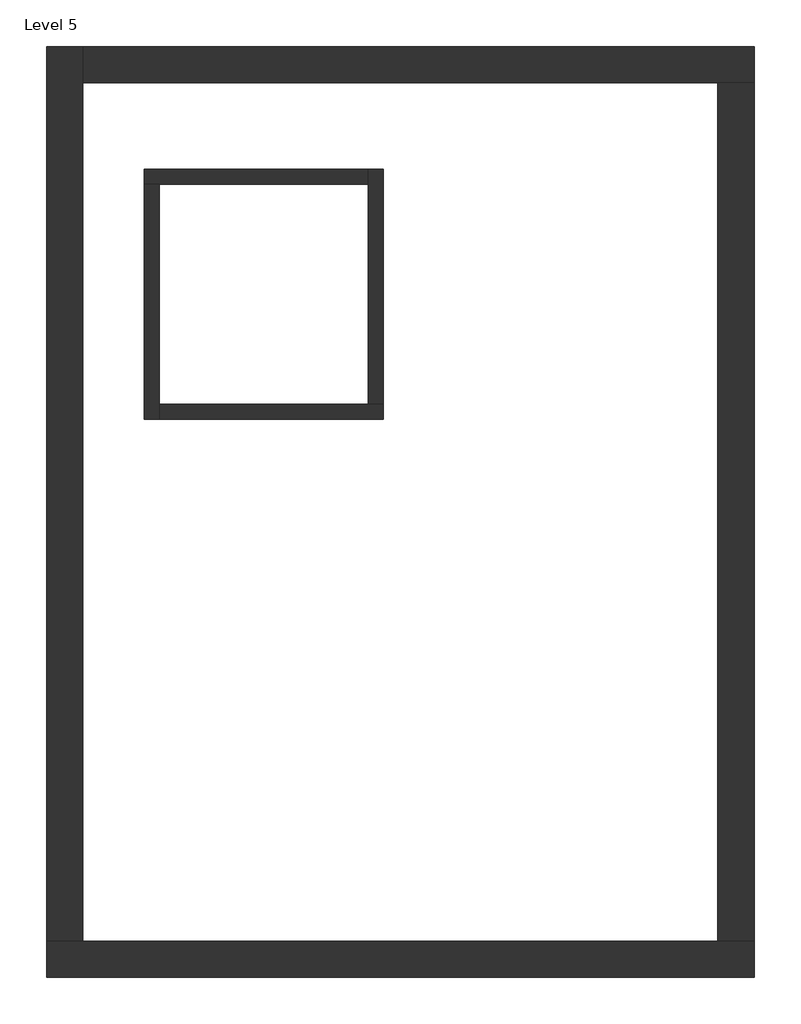
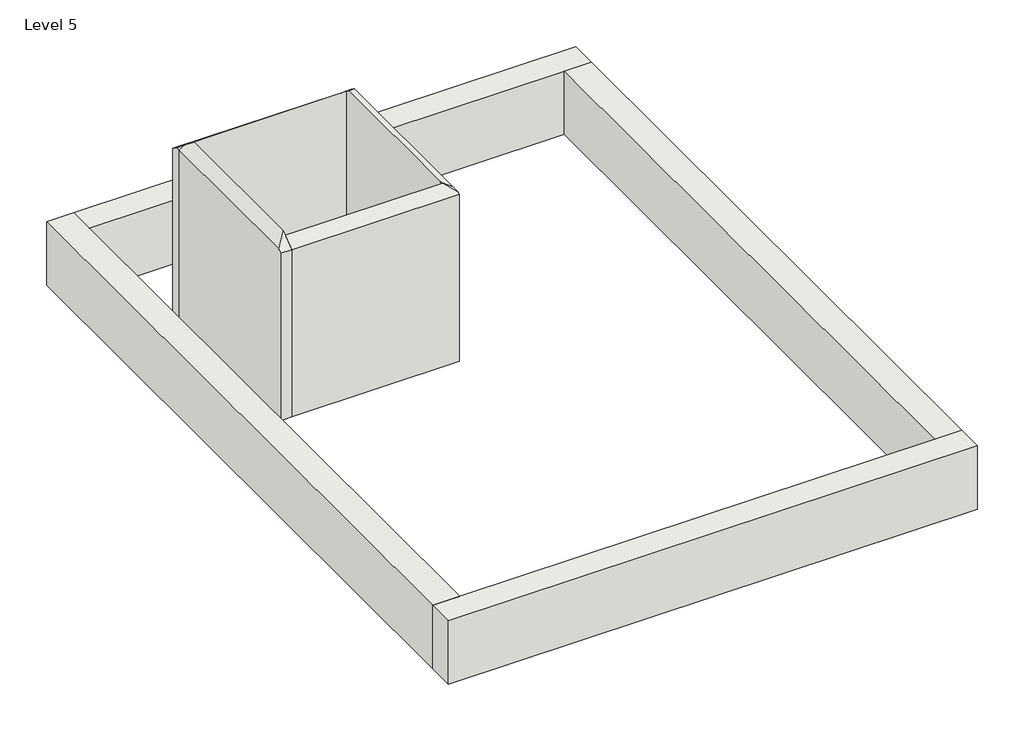
# One storey: 8 walls.
"""IFC4 building model written with IfcOpenShell, lengths in millimetres."""

from ifc_helpers import new_model, si_unit, frame, origin, place, context, project, spatial, polyline, outline, extrude, faceted_brep, element, save

model = new_model("IFC4")

# Units and contexts
model_context = context("Model", 3, world=origin())
ifc_project = project(units=[si_unit("LENGTHUNIT", "METRE", prefix="MILLI")], contexts=[model_context])

# Site, building, storey
site = spatial("IfcSite", under=ifc_project)
building = spatial("IfcBuilding", under=site)
storey = spatial("IfcBuildingStorey", under=building, Name="Level 5", Elevation=6553.2)

# Walls
placement = place(None, origin())
element("IfcWall", 1, ObjectType="Exterior - Brick on CMU", at=placement, inside=storey, context=model_context, shape_type="Brep", body=[
    faceted_brep([(-1013.5628458, 2205.3847306, 6553.2), (-1508.8628458, 2205.3847306, 6553.2), (-10157.5628458, 2205.3847306, 6553.2), (-10652.8628458, 2205.3847306, 6553.2), (-10652.8628458, 2205.3847306, 7772.4), (-10157.5628458, 2205.3847306, 7772.4), (-1508.8628458, 2205.3847306, 7772.4), (-1013.5628458, 2205.3847306, 7772.4), (-1013.5628458, 1710.0847306, 6553.2), (-1013.5628458, 1710.0847306, 7772.4), (-10652.8628458, 1710.0847306, 7772.4), (-10652.8628458, 1710.0847306, 6553.2)], [[[0, 1, 2, 3, 4, 5, 6, 7]], [[8, 9, 10, 11]], [[3, 2, 1, 0, 8, 11]], [[7, 6, 5, 4, 10, 9]], [[4, 3, 11, 10]], [[0, 7, 9, 8]]]),
])
element("IfcWall", 2, ObjectType="Exterior - Brick on CMU", at=placement, inside=storey, context=model_context, shape_type="Brep", body=[
    faceted_brep([(-10157.5628458, 2205.3847306, 6553.2), (-10157.5628458, 13897.569734, 6553.2), (-10157.5628458, 14392.869734, 6553.2), (-10157.5628458, 14392.869734, 7772.4), (-10157.5628458, 13897.569734, 7772.4), (-10157.5628458, 2205.3847306, 7772.4), (-10652.8628458, 2205.3847306, 6553.2), (-10652.8628458, 2205.3847306, 7772.4), (-10652.8628458, 14392.869734, 7772.4), (-10652.8628458, 14392.869734, 6553.2)], [[[0, 1, 2, 3, 4, 5]], [[6, 7, 8, 9]], [[2, 1, 0, 6, 9]], [[5, 4, 3, 8, 7]], [[0, 5, 7, 6]], [[3, 2, 9, 8]]]),
])
element("IfcWall", 3, ObjectType="Exterior - Brick on CMU", at=placement, inside=storey, context=model_context, shape_type="Brep", body=[
    faceted_brep([(-10157.5628458, 13897.569734, 6553.2), (-1508.8628458, 13897.569734, 6553.2), (-1013.5628458, 13897.569734, 6553.2), (-1013.5628458, 13897.569734, 7772.4), (-1508.8628458, 13897.569734, 7772.4), (-10157.5628458, 13897.569734, 7772.4), (-10157.5628458, 14392.869734, 6553.2), (-10157.5628458, 14392.869734, 7772.4), (-1013.5628458, 14392.869734, 7772.4), (-1013.5628458, 14392.869734, 6553.2)], [[[0, 1, 2, 3, 4, 5]], [[6, 7, 8, 9]], [[2, 1, 0, 6, 9]], [[5, 4, 3, 8, 7]], [[0, 5, 7, 6]], [[3, 2, 9, 8]]]),
])
element("IfcWall", 4, ObjectType="Exterior - Brick on CMU", at=placement, inside=storey, context=model_context, shape_type="SweptSolid", body=[
    extrude(outline(polyline([(-1508.8628458, 2205.3847306), (-1508.8628458, 13897.569734), (-1013.5628458, 13897.569734), (-1013.5628458, 2205.3847306), (-1508.8628458, 2205.3847306)])), frame((0.0, 0.0, 6553.2), z_axis=(0.0, 0.0, 1.0), x_axis=(1.0, 0.0, 0.0)), (0.0, 0.0, 1.0), 1219.2),
])
element("IfcWall", 5, ObjectType="Generic - 8\"", at=placement, inside=storey, context=model_context, shape_type="Brep", body=[
    faceted_brep([(-9318.8651458, 12517.3039814, 6553.2), (-9115.6651458, 12517.3039814, 6553.2), (-6270.8651458, 12517.3039814, 6553.2), (-6270.8651458, 12517.3039814, 9884.5570213), (-9115.6651458, 12517.3039814, 9884.5570213), (-9234.8498885, 12517.3039814, 9884.5570213), (-9318.8651458, 12517.3039814, 9821.5455782), (-9318.8651458, 12720.5039814, 6553.2), (-9318.8651458, 12720.5039814, 9732.1570213), (-6270.8651458, 12720.5039814, 9732.1570213), (-6270.8651458, 12720.5039814, 6553.2), (-9318.8651458, 12601.3192387, 9821.5455782)], [[[0, 1, 2, 3, 4, 5, 6]], [[7, 8, 9, 10]], [[2, 1, 0, 7, 10]], [[0, 6, 11, 8, 7]], [[3, 2, 10, 9]], [[6, 5, 11]], [[5, 4, 3, 9, 8, 11]]]),
])
element("IfcWall", 6, ObjectType="Generic - 8\"", at=placement, inside=storey, context=model_context, shape_type="Brep", body=[
    faceted_brep([(-9115.6651458, 9316.9039814, 6553.2), (-9115.6651458, 9520.1039814, 6553.2), (-9115.6651458, 12517.3039814, 6553.2), (-9115.6651458, 12517.3039814, 9884.5570213), (-9115.6651458, 12398.1192387, 9973.9455782), (-9115.6651458, 9582.1074474, 9973.9455782), (-9115.6651458, 9520.1039814, 9927.4429787), (-9115.6651458, 9316.9039814, 9775.0429787), (-9318.8651458, 9316.9039814, 6553.2), (-9318.8651458, 9316.9039814, 9775.0429787), (-9318.8651458, 9378.9074474, 9821.5455782), (-9318.8651458, 12517.3039814, 9821.5455782), (-9318.8651458, 12517.3039814, 6553.2), (-9234.8498885, 12517.3039814, 9884.5570213)], [[[0, 1, 2, 3, 4, 5, 6, 7]], [[8, 9, 10, 11, 12]], [[2, 1, 0, 8, 12]], [[0, 7, 9, 8]], [[3, 2, 12, 11, 13]], [[7, 6, 5, 10, 9]], [[5, 4, 13, 11, 10]], [[4, 3, 13]]]),
])
element("IfcWall", 7, ObjectType="Generic - 8\"", at=placement, inside=storey, context=model_context, shape_type="Brep", body=[
    faceted_brep([(-6067.6651458, 9520.1039814, 6553.2), (-6270.8651458, 9520.1039814, 6553.2), (-9115.6651458, 9520.1039814, 6553.2), (-9115.6651458, 9520.1039814, 9927.4429787), (-6270.8651458, 9520.1039814, 9927.4429787), (-6237.6498885, 9520.1039814, 9927.4429787), (-6067.6651458, 9520.1039814, 9799.9544218), (-6067.6651458, 9316.9039814, 6553.2), (-6067.6651458, 9316.9039814, 9775.0429787), (-9115.6651458, 9316.9039814, 9775.0429787), (-9115.6651458, 9316.9039814, 6553.2), (-6067.6651458, 9350.1192387, 9799.9544218)], [[[0, 1, 2, 3, 4, 5, 6]], [[7, 8, 9, 10]], [[2, 1, 0, 7, 10]], [[0, 6, 11, 8, 7]], [[3, 2, 10, 9]], [[6, 5, 11]], [[5, 4, 3, 9, 8, 11]]]),
])
element("IfcWall", 8, ObjectType="Generic - 8\"", at=placement, inside=storey, context=model_context, shape_type="Brep", body=[
    faceted_brep([(-6270.8651458, 12720.5039814, 6553.2), (-6270.8651458, 12517.3039814, 6553.2), (-6270.8651458, 9520.1039814, 6553.2), (-6270.8651458, 9520.1039814, 9927.4429787), (-6270.8651458, 9553.3192387, 9952.3544218), (-6270.8651458, 12426.9074474, 9952.3544218), (-6270.8651458, 12517.3039814, 9884.5570213), (-6270.8651458, 12720.5039814, 9732.1570213), (-6067.6651458, 12720.5039814, 6553.2), (-6067.6651458, 12720.5039814, 9732.1570213), (-6067.6651458, 12630.1074474, 9799.9544218), (-6067.6651458, 9520.1039814, 9799.9544218), (-6067.6651458, 9520.1039814, 6553.2), (-6237.6498885, 9520.1039814, 9927.4429787)], [[[0, 1, 2, 3, 4, 5, 6, 7]], [[8, 9, 10, 11, 12]], [[2, 1, 0, 8, 12]], [[0, 7, 9, 8]], [[3, 2, 12, 11, 13]], [[7, 6, 5, 10, 9]], [[5, 4, 13, 11, 10]], [[4, 3, 13]]]),
])

save(model, "model.ifc")

# Revit data of these elements
# Type "Exterior - Brick on CMU"
#   Assembly Code = "B2010156"
#   Layers, outside or top first: 0' - 3 5/8" "Brick, Common" (function 4); 0' - 3" "Air" (function 3); 0' - 3" "Rigid insulation" (function 3); 0' - 0" "Damp-proofing" (function 100); 0' - 7 5/8" "Concrete Masonry Units" (function 1); 0' - 1 5/8" "Metal Furring" (function 2); 0' - 0 5/8" "Gypsum Wall Board" (function 5)
# Type "Generic - 8\""
#   Assembly Code = "B2010"
#   Layers, outside or top first: 0' - 8" no material (function 1)
# Element 1 (IfcWall, "Exterior - Brick on CMU")
#   Top Offset = 0' - 0"
#   Base Offset = 0' - 0"
#   Unconnected Height = 4' - 0"
#   wall height = 4' - 0"
#   Phase Created = New Construction
#   Base Constraint = Level 5
#   Materials on its faces: "Brick, Common", "Default Wall", "Gypsum Wall Board"
# Elements 2, 3 (IfcWall, "Exterior - Brick on CMU")
#   Top Offset = 0' - 0"
#   Base Offset = 0' - 0"
#   Unconnected Height = 4' - 0"
#   wall height = 4' - 0"
#   Phase Created = New Construction
#   Base Constraint = Level 5
#   Materials on its faces: "Default Wall", "Brick, Common", "Gypsum Wall Board"
# Element 4 (IfcWall, "Exterior - Brick on CMU")
#   Top Offset = 0' - 0"
#   Base Offset = 0' - 0"
#   Unconnected Height = 4' - 0"
#   wall height = 4' - 0"
#   Phase Created = New Construction
#   Base Constraint = Level 5
#   Materials on its faces: "Default Wall", "Gypsum Wall Board", "Brick, Common"
# Elements 5, 6, 7, 8 (IfcWall, "Generic - 8\"")
#   Top Offset = 0' - 0"
#   Base Offset = 0' - 0"
#   Unconnected Height = 10' - 0"
#   wall height = 10' - 0"
#   Phase Created = New Construction
#   Base Constraint = Level 5
#   Materials on its faces: "Default Wall"
# Materials
#   "Brick, Common": class "Masonry", colour RGB 170 98 104, transparency 0, Description = "Common brick", Cost = 0
#   "Air": class "Gas", colour RGB 255 255 255, transparency 0, Description = "Air", Cost = 0
#   "Rigid insulation": class "Generic", colour RGB 127 127 127, transparency 0, Description = "Rigid foam insulation board", Cost = 0
#   "Damp-proofing": class "Generic", colour RGB 127 127 127, transparency 0, Description = "Damp-proofing", Cost = 0
#   "Concrete Masonry Units": class "Masonry", colour RGB 227 227 227, transparency 0, Description = "Concrete masonry units", Cost = 0
#   "Metal Furring": class "Metal", colour RGB 199 199 199, transparency 0, Description = "Light gauge steel furring", Cost = 0
#   "Gypsum Wall Board": class "Generic", colour RGB 127 127 127, transparency 0, Description = "Gypsum Wall Board", Cost = 0
#   "Default Wall": colour RGB 128 128 128, transparency 0
